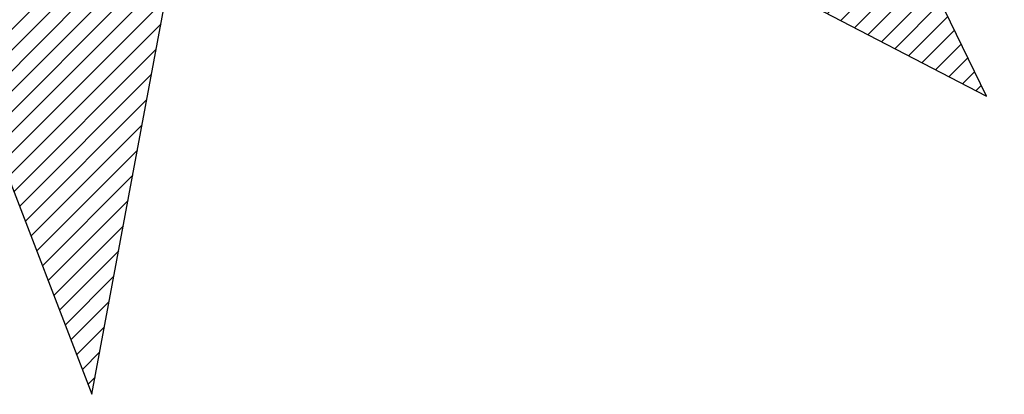
# Model space of a CAD drawing. Units: inches. Extents: x 1986 to 21484, y -1816 to 2016.
# Tile 25 of 85: x 2172.01 to 2182.45, y 1865.09 to 1869.06. Entities that reach past the tile are written whole.
import ezdxf

# ---------------------------------------------------------------- set-up
doc = ezdxf.new("R2010")
doc.units = ezdxf.units.IN
doc.layers.add('L-PLNT', color=84, linetype='Continuous', lineweight=13)
doc.layers.add('vfolhas', color=114, linetype='Continuous', lineweight=5)
doc.layers.add('vfolha', color=72, linetype='Continuous')
doc.layers.add('vfolhas2', color=102, linetype='Continuous')
pattern_1 = [(45, (-2446.5133113, 50.986076), (-0.004419417382, 0.004419417382), [])]

# ---------------------------------------------------------------- blocks, each defined once
blk = doc.blocks.new('arbusto_PB_verde_grande')
at = {"layer": 'vfolhas'}
h = blk.add_hatch(dxfattribs=at)
h.set_pattern_fill('ANSI31', color=256, scale=0.05, style=0)
h.set_pattern_definition(pattern_1)
h.paths.add_polyline_path([(-0.07279, 0.50669), (-0.18085, 0.65063), (-0.2334, 0.67253), (-0.20712, 0.53176), (-0.10785, 0.25007), (0.02625, -0.03934), (0.00028, 0.09048), (0.00816, 0.16241), (-0.04939, 0.29079)])
h.paths.add_polyline_path([(0.09902, 0.41929), (0.09372, 0.26573), (0.07906, 0.18814), (0.15506, 0.36901), (0.26606, 0.5505), (0.28356, 0.63504), (0.2485, 0.68819), (0.25145, 0.63504), (0.20178, 0.54426)])
h.paths.add_polyline_path([(0.12295, 0.24073), (0.047, 0.06233), (0.02625, -0.03934), (0.11122, 0.04358), (0.18428, 0.09364), (0.27478, 0.19376), (0.3215, 0.25323), (0.44129, 0.38467), (0.47634, 0.57866), (0.41789, 0.45347), (0.28939, 0.30954)])
h.paths.add_polyline_path([(0.58145, -0.03779), (0.70707, 0.01536), (0.78591, 0.04667), (0.74796, 0.06549), (0.62818, 0.08423), (0.52595, 0.09048), (0.39745, 0.04358), (0.02625, -0.03934), (0.25728, -0.03154), (0.43834, -0.0347)])
h.paths.add_polyline_path([(0.52022, -0.03647), (0.43834, -0.0347), (0.25728, -0.03154), (0.02625, -0.03934), (0.17964, -0.08515), (0.53768, -0.13167), (0.69541, -0.15357), (0.78591, -0.07852), (0.70413, -0.10042)])
h.paths.add_polyline_path([(0.27189, -0.21929), (0.14922, -0.14107), (0.02625, -0.03934), (0.15794, -0.31007), (0.29522, -0.42585), (0.41789, -0.49157), (0.56396, -0.56669), (0.5114, -0.48532), (0.39456, -0.34139)])
h.paths.add_polyline_path([(-0.05818, -0.47591), (-0.02312, -0.61984), (0.047, -0.80134), (0.08494, -0.59794), (0.07911, -0.4071), (0.03527, -0.25376), (0.02625, -0.03934), (-0.03773, -0.26001)])
h.paths.add_polyline_path([(-0.24218, 0.14054), (-0.11073, 0.06858), (0.02625, -0.03934), (-0.04235, 0.10871), (-0.21007, 0.23757), (-0.36485, 0.33145), (-0.47874, 0.40341), (-0.54303, 0.46288), (-0.49041, 0.33145), (-0.39408, 0.22192)])
h = blk.add_hatch(dxfattribs=at)
h.set_pattern_fill('ANSI31', color=256, scale=0.05, style=0)
h.set_pattern_definition(pattern_1)
h.paths.add_polyline_path([(0.33611, -0.623), (0.43251, -0.67306), (0.39456, -0.59485), (0.3303, -0.44464), (0.29522, -0.42585), (0.15794, -0.31007), (0.14904, -0.29177), (0.18428, -0.44151)])
at = {"layer": 'vfolha'}
for p, q in [((0.047, -0.80134), (0.08494, -0.59794)), ((-0.02312, -0.61984), (0.047, -0.80134))]:
    blk.add_line(p, q, dxfattribs=at)
at = {"layer": 'vfolhas2'}
for p, q in [((0.43251, -0.67306), (0.39456, -0.59485)), ((0.33611, -0.623), (0.43251, -0.67306))]:
    blk.add_line(p, q, dxfattribs=at)

msp = doc.modelspace()

# ---------------------------------------------------------------- block references
at = {"layer": 'L-PLNT', "xscale": 24.60366729364114, "yscale": 24.60366729364114, "zscale": 24.60366729364114}
msp.add_blockref('arbusto_PB_verde_grande', (2171.623, 1884.805), dxfattribs=at)

doc.saveas('drawing.dxf')
